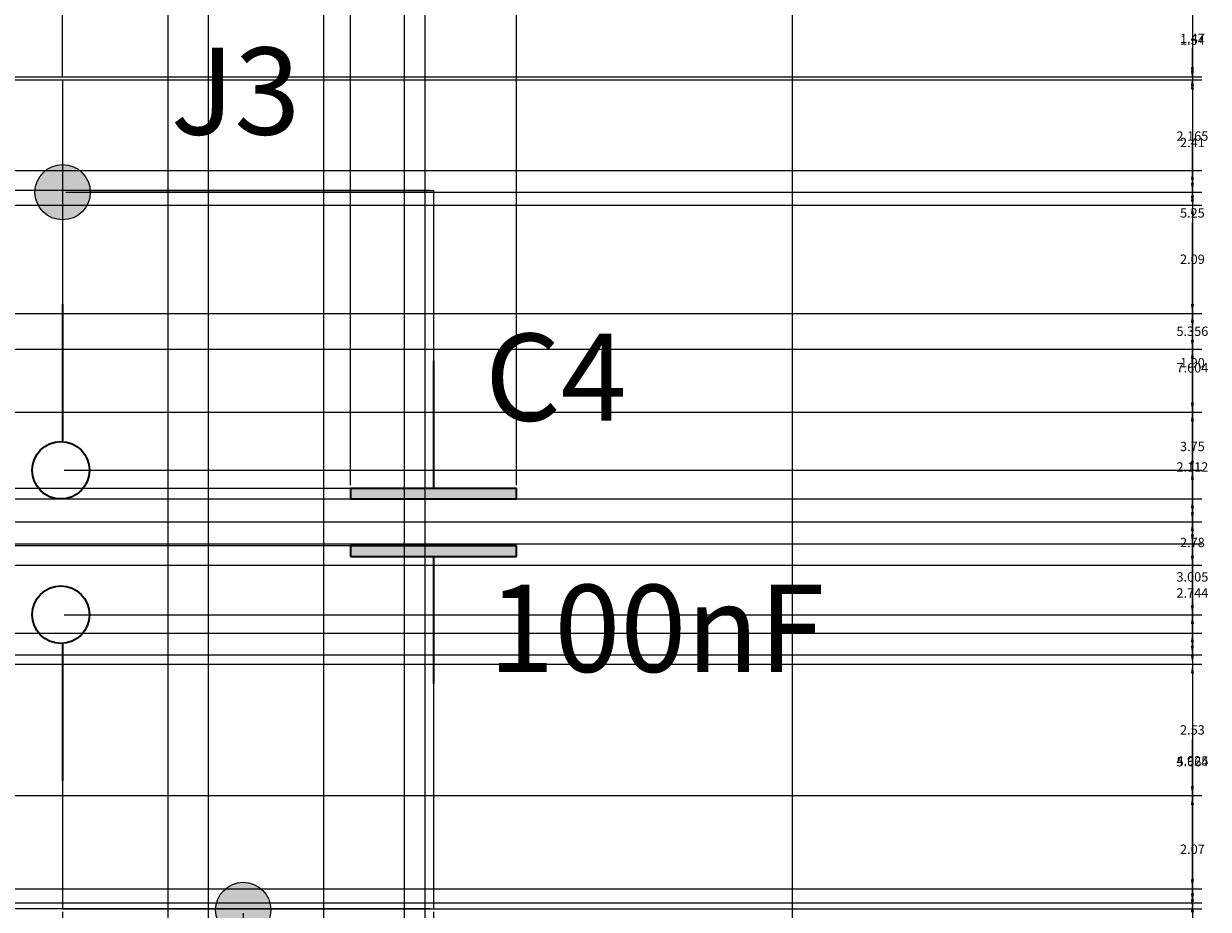
# Model space of a CAD drawing. Units: inches. Extents: x 23 to 132, y 5 to 105.
# Tile 12 of 14: x 106.54 to 129.37, y 59.58 to 76.64. Entities that reach past the tile are written whole.
import ezdxf

# ---------------------------------------------------------------- set-up
doc = ezdxf.new("R2010")
doc.units = ezdxf.units.IN
doc.header["$MEASUREMENT"] = 0
for name, color, linetype, lineweight in [('A-ANNO-DIMS', 2, 'Continuous', 18), ('E-ANNO-IDEN', 4, 'Continuous', 18), ('E-SYMB', 1, 'Continuous', 35), ('E-SYMB-PATT', 1, 'Continuous', 18), ('E-WIRE', 3, 'Continuous', 25), ('E-WIRE-PATT', 3, 'Continuous', 18)]:
    doc.layers.add(name, color=color, linetype=linetype, lineweight=lineweight)
doc.styles.get("Standard").update_dxf_attribs({"font": 'arial.ttf'})
doc.dimstyles.get("Standard").update_dxf_attribs({"dimtxt": 0.18, "dimasz": 0.18, "dimexe": 0.18, "dimexo": 0.0625, "dimgap": 0.09, "dimtad": 0, "dimtih": 1, "dimtoh": 1, "dimdec": 4, "dimzin": 0, "dimdsep": 46, "dimtxsty": 'Standard', "dimcen": 0.09, "dimadec": 0, "dimazin": 0, "dimtfac": 1, "dimtdec": 4, "dimtofl": 0, "dimtmove": 0, "dimatfit": 3, "dimfxl": 1, "dimtolj": 1, "dimtzin": 0, "dimarcsym": 0})

# ---------------------------------------------------------------- blocks, each defined once
blk = doc.blocks.new('*D2')
at = {"layer": 'A-ANNO-DIMS', "color": 0, "lineweight": -2, "transparency": 16777216}
for p, q in [((28.697, 66.272), (28.697, 105.232)), ((28.877, 105.052), (75.577, 105.052)), ((123.031, 105.052), (76.33, 105.052)), ((123.211, 99.539), (123.211, 105.232))]:
    blk.add_line(p, q, dxfattribs=at)
at = {"layer": 'A-ANNO-DIMS', "color": 0, "transparency": 16777216}
for points in [[(28.877, 105.082), (28.877, 105.022), (28.697, 105.052)], [(123.031, 105.082), (123.031, 105.022), (123.211, 105.052)]]:
    blk.add_solid(points, dxfattribs=at)
at = {"layer": 'Defpoints', "color": 0, "transparency": 16777216}
for p in [(123.211, 105.052), (123.211, 99.477), (28.697, 66.21)]:
    blk.add_point(p, dxfattribs=at)
at = {"layer": 'A-ANNO-DIMS', "color": 0, "transparency": 16777216, "insert": (75.954, 105.052), "char_height": 0.18, "attachment_point": 5}
blk.add_mtext('\\A1;94.51', dxfattribs=at)
blk = doc.blocks.new('*D3')
at = {"layer": 'A-ANNO-DIMS', "color": 0, "lineweight": -2, "transparency": 16777216}
for p, q in [((121.409, 99.285), (129.239, 99.285)), ((129.059, 99.105), (129.059, 55.423)), ((129.059, 11.378), (129.059, 55.06)), ((72.981, 11.198), (129.239, 11.198))]:
    blk.add_line(p, q, dxfattribs=at)
at = {"layer": 'A-ANNO-DIMS', "color": 0, "transparency": 16777216}
for points in [[(129.029, 99.105), (129.089, 99.105), (129.059, 99.285)], [(129.029, 11.378), (129.089, 11.378), (129.059, 11.198)]]:
    blk.add_solid(points, dxfattribs=at)
at = {"layer": 'Defpoints', "color": 0, "transparency": 16777216}
for p in [(121.346, 99.285), (129.059, 99.285), (72.919, 11.198)]:
    blk.add_point(p, dxfattribs=at)
at = {"layer": 'A-ANNO-DIMS', "color": 0, "transparency": 16777216, "insert": (129.059, 55.241), "char_height": 0.18, "attachment_point": 5}
blk.add_mtext('\\A1;88.09', dxfattribs=at)
blk = doc.blocks.new('*D15')
at = {"layer": 'A-ANNO-DIMS', "color": 0, "lineweight": -2, "transparency": 16777216}
for p, q in [((50.327, 77.095), (129.239, 77.095)), ((129.059, 76.915), (129.059, 76.538)), ((129.059, 75.801), (129.059, 76.177)), ((47.783, 75.621), (129.239, 75.621))]:
    blk.add_line(p, q, dxfattribs=at)
at = {"layer": 'A-ANNO-DIMS', "color": 0, "transparency": 16777216}
for points in [[(129.029, 76.915), (129.089, 76.915), (129.059, 77.095)], [(129.029, 75.801), (129.089, 75.801), (129.059, 75.621)]]:
    blk.add_solid(points, dxfattribs=at)
at = {"layer": 'Defpoints', "color": 0, "transparency": 16777216}
for p in [(50.265, 77.095), (47.72, 75.621), (129.059, 75.621)]:
    blk.add_point(p, dxfattribs=at)
at = {"layer": 'A-ANNO-DIMS', "color": 0, "transparency": 16777216, "insert": (129.059, 76.358), "char_height": 0.18, "attachment_point": 5}
blk.add_mtext('\\A1;1.47', dxfattribs=at)
blk = doc.blocks.new('*D16')
at = {"layer": 'A-ANNO-DIMS', "color": 0, "lineweight": -2, "transparency": 16777216}
for p, q in [((47.783, 75.621), (129.239, 75.621)), ((129.059, 75.441), (129.059, 73.177)), ((129.059, 70.55), (129.059, 72.814)), ((47.783, 70.37), (129.239, 70.37))]:
    blk.add_line(p, q, dxfattribs=at)
at = {"layer": 'A-ANNO-DIMS', "color": 0, "transparency": 16777216}
for points in [[(129.029, 75.441), (129.089, 75.441), (129.059, 75.621)], [(129.029, 70.55), (129.089, 70.55), (129.059, 70.37)]]:
    blk.add_solid(points, dxfattribs=at)
at = {"layer": 'Defpoints', "color": 0, "transparency": 16777216}
for p in [(47.72, 75.621), (47.72, 70.37), (129.059, 70.37)]:
    blk.add_point(p, dxfattribs=at)
at = {"layer": 'A-ANNO-DIMS', "color": 0, "transparency": 16777216, "insert": (129.059, 72.996), "char_height": 0.18, "attachment_point": 5}
blk.add_mtext('\\A1;5.25', dxfattribs=at)
blk = doc.blocks.new('*D17')
at = {"layer": 'A-ANNO-DIMS', "color": 0, "lineweight": -2, "transparency": 16777216}
for p, q in [((47.783, 70.37), (129.239, 70.37)), ((129.059, 70.19), (129.059, 68.678)), ((129.059, 66.801), (129.059, 68.314)), ((47.783, 66.621), (129.239, 66.621))]:
    blk.add_line(p, q, dxfattribs=at)
at = {"layer": 'A-ANNO-DIMS', "color": 0, "transparency": 16777216}
for points in [[(129.029, 70.19), (129.089, 70.19), (129.059, 70.37)], [(129.029, 66.801), (129.089, 66.801), (129.059, 66.621)]]:
    blk.add_solid(points, dxfattribs=at)
at = {"layer": 'Defpoints', "color": 0, "transparency": 16777216}
for p in [(47.72, 70.37), (47.72, 66.621), (129.059, 66.621)]:
    blk.add_point(p, dxfattribs=at)
at = {"layer": 'A-ANNO-DIMS', "color": 0, "transparency": 16777216, "insert": (129.059, 68.496), "char_height": 0.18, "attachment_point": 5}
blk.add_mtext('\\A1;3.75', dxfattribs=at)
blk = doc.blocks.new('*D24')
at = {"layer": 'A-ANNO-DIMS', "color": 0, "lineweight": -2, "transparency": 16777216}
for p, q in [((81.032, 77.095), (129.239, 77.095)), ((129.059, 76.915), (129.059, 76.509)), ((129.059, 75.739), (129.059, 76.145)), ((83.576, 75.559), (129.239, 75.559))]:
    blk.add_line(p, q, dxfattribs=at)
at = {"layer": 'A-ANNO-DIMS', "color": 0, "transparency": 16777216}
for points in [[(129.029, 76.915), (129.089, 76.915), (129.059, 77.095)], [(129.029, 75.739), (129.089, 75.739), (129.059, 75.559)]]:
    blk.add_solid(points, dxfattribs=at)
at = {"layer": 'Defpoints', "color": 0, "transparency": 16777216}
for p in [(80.969, 77.095), (83.514, 75.559), (129.059, 75.559)]:
    blk.add_point(p, dxfattribs=at)
at = {"layer": 'A-ANNO-DIMS', "color": 0, "transparency": 16777216, "insert": (129.059, 76.327), "char_height": 0.18, "attachment_point": 5}
blk.add_mtext('\\A1;1.54', dxfattribs=at)
blk = doc.blocks.new('*D25')
at = {"layer": 'A-ANNO-DIMS', "color": 0, "lineweight": -2, "transparency": 16777216}
for p, q in [((83.576, 75.559), (129.239, 75.559)), ((129.059, 75.379), (129.059, 74.534)), ((129.059, 73.327), (129.059, 74.173)), ((83.576, 73.147), (129.239, 73.147))]:
    blk.add_line(p, q, dxfattribs=at)
at = {"layer": 'A-ANNO-DIMS', "color": 0, "transparency": 16777216}
for points in [[(129.029, 75.379), (129.089, 75.379), (129.059, 75.559)], [(129.029, 73.327), (129.089, 73.327), (129.059, 73.147)]]:
    blk.add_solid(points, dxfattribs=at)
at = {"layer": 'Defpoints', "color": 0, "transparency": 16777216}
for p in [(83.514, 75.559), (83.514, 73.147), (129.059, 73.147)]:
    blk.add_point(p, dxfattribs=at)
at = {"layer": 'A-ANNO-DIMS', "color": 0, "transparency": 16777216, "insert": (129.059, 74.353), "char_height": 0.18, "attachment_point": 5}
blk.add_mtext('\\A1;2.41', dxfattribs=at)
blk = doc.blocks.new('*D26')
at = {"layer": 'A-ANNO-DIMS', "color": 0, "lineweight": -2, "transparency": 16777216}
for p, q in [((83.576, 73.147), (129.239, 73.147)), ((129.059, 72.967), (129.059, 72.286)), ((129.059, 71.241), (129.059, 71.922)), ((83.576, 71.061), (129.239, 71.061))]:
    blk.add_line(p, q, dxfattribs=at)
at = {"layer": 'A-ANNO-DIMS', "color": 0, "transparency": 16777216}
for points in [[(129.029, 72.967), (129.089, 72.967), (129.059, 73.147)], [(129.029, 71.241), (129.089, 71.241), (129.059, 71.061)]]:
    blk.add_solid(points, dxfattribs=at)
at = {"layer": 'Defpoints', "color": 0, "transparency": 16777216}
for p in [(83.514, 73.147), (83.514, 71.061), (129.059, 71.061)]:
    blk.add_point(p, dxfattribs=at)
at = {"layer": 'A-ANNO-DIMS', "color": 0, "transparency": 16777216, "insert": (129.059, 72.104), "char_height": 0.18, "attachment_point": 5}
blk.add_mtext('\\A1;2.09', dxfattribs=at)
blk = doc.blocks.new('*D27')
at = {"layer": 'A-ANNO-DIMS', "color": 0, "lineweight": -2, "transparency": 16777216}
for p, q in [((83.576, 71.061), (129.239, 71.061)), ((129.059, 70.881), (129.059, 70.292)), ((129.059, 69.338), (129.059, 69.928)), ((83.576, 69.158), (129.239, 69.158))]:
    blk.add_line(p, q, dxfattribs=at)
at = {"layer": 'A-ANNO-DIMS', "color": 0, "transparency": 16777216}
for points in [[(129.029, 70.881), (129.089, 70.881), (129.059, 71.061)], [(129.029, 69.338), (129.089, 69.338), (129.059, 69.158)]]:
    blk.add_solid(points, dxfattribs=at)
at = {"layer": 'Defpoints', "color": 0, "transparency": 16777216}
for p in [(83.514, 71.061), (83.514, 69.158), (129.059, 69.158)]:
    blk.add_point(p, dxfattribs=at)
at = {"layer": 'A-ANNO-DIMS', "color": 0, "transparency": 16777216, "insert": (129.059, 70.11), "char_height": 0.18, "attachment_point": 5}
blk.add_mtext('\\A1;1.90', dxfattribs=at)
blk = doc.blocks.new('*D28')
at = {"layer": 'A-ANNO-DIMS', "color": 0, "lineweight": -2, "transparency": 16777216}
for p, q in [((83.576, 69.158), (129.239, 69.158)), ((129.059, 68.978), (129.059, 68.282)), ((129.059, 67.226), (129.059, 67.922)), ((83.576, 67.046), (129.239, 67.046))]:
    blk.add_line(p, q, dxfattribs=at)
at = {"layer": 'A-ANNO-DIMS', "color": 0, "transparency": 16777216}
for points in [[(129.029, 68.978), (129.089, 68.978), (129.059, 69.158)], [(129.029, 67.226), (129.089, 67.226), (129.059, 67.046)]]:
    blk.add_solid(points, dxfattribs=at)
at = {"layer": 'Defpoints', "color": 0, "transparency": 16777216}
for p in [(83.514, 69.158), (83.514, 67.046), (129.059, 67.046)]:
    blk.add_point(p, dxfattribs=at)
at = {"layer": 'A-ANNO-DIMS', "color": 0, "transparency": 16777216, "insert": (129.059, 68.102), "char_height": 0.18, "attachment_point": 5}
blk.add_mtext('\\A1;2.112', dxfattribs=at)
blk = doc.blocks.new('*D29')
at = {"layer": 'A-ANNO-DIMS', "color": 0, "lineweight": -2, "transparency": 16777216}
for p, q in [((83.576, 67.046), (129.239, 67.046)), ((129.059, 66.866), (129.059, 65.855)), ((129.059, 64.482), (129.059, 65.494)), ((83.576, 64.302), (129.239, 64.302))]:
    blk.add_line(p, q, dxfattribs=at)
at = {"layer": 'A-ANNO-DIMS', "color": 0, "transparency": 16777216}
for points in [[(129.029, 66.866), (129.089, 66.866), (129.059, 67.046)], [(129.029, 64.482), (129.089, 64.482), (129.059, 64.302)]]:
    blk.add_solid(points, dxfattribs=at)
at = {"layer": 'Defpoints', "color": 0, "transparency": 16777216}
for p in [(83.514, 67.046), (83.514, 64.302), (129.059, 64.302)]:
    blk.add_point(p, dxfattribs=at)
at = {"layer": 'A-ANNO-DIMS', "color": 0, "transparency": 16777216, "insert": (129.059, 65.674), "char_height": 0.18, "attachment_point": 5}
blk.add_mtext('\\A1;2.744', dxfattribs=at)
blk = doc.blocks.new('*D30')
at = {"layer": 'A-ANNO-DIMS', "color": 0, "lineweight": -2, "transparency": 16777216}
for p, q in [((83.576, 64.302), (129.239, 64.302)), ((129.059, 64.122), (129.059, 63.217)), ((129.059, 61.949), (129.059, 62.853)), ((83.576, 61.769), (129.239, 61.769))]:
    blk.add_line(p, q, dxfattribs=at)
at = {"layer": 'A-ANNO-DIMS', "color": 0, "transparency": 16777216}
for points in [[(129.029, 64.122), (129.089, 64.122), (129.059, 64.302)], [(129.029, 61.949), (129.089, 61.949), (129.059, 61.769)]]:
    blk.add_solid(points, dxfattribs=at)
at = {"layer": 'Defpoints', "color": 0, "transparency": 16777216}
for p in [(83.514, 64.302), (83.514, 61.769), (129.059, 61.769)]:
    blk.add_point(p, dxfattribs=at)
at = {"layer": 'A-ANNO-DIMS', "color": 0, "transparency": 16777216, "insert": (129.059, 63.035), "char_height": 0.18, "attachment_point": 5}
blk.add_mtext('\\A1;2.53', dxfattribs=at)
blk = doc.blocks.new('*D31')
at = {"layer": 'A-ANNO-DIMS', "color": 0, "lineweight": -2, "transparency": 16777216}
for p, q in [((83.576, 61.769), (129.239, 61.769)), ((129.059, 61.589), (129.059, 60.918)), ((129.059, 59.883), (129.059, 60.554)), ((83.576, 59.703), (129.239, 59.703))]:
    blk.add_line(p, q, dxfattribs=at)
at = {"layer": 'A-ANNO-DIMS', "color": 0, "transparency": 16777216}
for points in [[(129.029, 61.589), (129.089, 61.589), (129.059, 61.769)], [(129.029, 59.883), (129.089, 59.883), (129.059, 59.703)]]:
    blk.add_solid(points, dxfattribs=at)
at = {"layer": 'Defpoints', "color": 0, "transparency": 16777216}
for p in [(83.514, 61.769), (83.514, 59.703), (129.059, 59.703)]:
    blk.add_point(p, dxfattribs=at)
at = {"layer": 'A-ANNO-DIMS', "color": 0, "transparency": 16777216, "insert": (129.059, 60.736), "char_height": 0.18, "attachment_point": 5}
blk.add_mtext('\\A1;2.07', dxfattribs=at)
blk = doc.blocks.new('*D32')
at = {"layer": 'A-ANNO-DIMS', "color": 0, "lineweight": -2, "transparency": 16777216}
for p, q in [((83.576, 59.703), (129.239, 59.703)), ((129.059, 59.523), (129.059, 58.629)), ((129.059, 57.372), (129.059, 58.266)), ((83.576, 57.192), (129.239, 57.192))]:
    blk.add_line(p, q, dxfattribs=at)
at = {"layer": 'A-ANNO-DIMS', "color": 0, "transparency": 16777216}
for points in [[(129.029, 59.523), (129.089, 59.523), (129.059, 59.703)], [(129.029, 57.372), (129.089, 57.372), (129.059, 57.192)]]:
    blk.add_solid(points, dxfattribs=at)
at = {"layer": 'Defpoints', "color": 0, "transparency": 16777216}
for p in [(83.514, 59.703), (83.514, 57.192), (129.059, 57.192)]:
    blk.add_point(p, dxfattribs=at)
at = {"layer": 'A-ANNO-DIMS', "color": 0, "transparency": 16777216, "insert": (129.059, 58.447), "char_height": 0.18, "attachment_point": 5}
blk.add_mtext('\\A1;2.51', dxfattribs=at)
blk = doc.blocks.new('*D49')
at = {"layer": 'A-ANNO-DIMS', "color": 0, "lineweight": -2, "transparency": 16777216}
for p, q in [((83.514, 75.622), (83.514, 105.232)), ((83.694, 105.052), (94.936, 105.052)), ((107.107, 105.052), (95.865, 105.052)), ((107.287, 75.622), (107.287, 105.232))]:
    blk.add_line(p, q, dxfattribs=at)
at = {"layer": 'A-ANNO-DIMS', "color": 0, "transparency": 16777216}
for points in [[(83.694, 105.082), (83.694, 105.022), (83.514, 105.052)], [(107.107, 105.082), (107.107, 105.022), (107.287, 105.052)]]:
    blk.add_solid(points, dxfattribs=at)
at = {"layer": 'Defpoints', "color": 0, "transparency": 16777216}
for p in [(107.287, 105.052), (83.514, 75.559), (107.287, 75.559)]:
    blk.add_point(p, dxfattribs=at)
at = {"layer": 'A-ANNO-DIMS', "color": 0, "transparency": 16777216, "insert": (95.4, 105.052), "char_height": 0.18, "attachment_point": 5}
blk.add_mtext('\\A1;23.774', dxfattribs=at)
blk = doc.blocks.new('*D57')
at = {"layer": 'A-ANNO-DIMS', "color": 0, "lineweight": -2, "transparency": 16777216}
for p, q in [((30.358, 64.901), (129.239, 64.901)), ((129.059, 64.721), (129.059, 62.62)), ((129.059, 60.155), (129.059, 62.256)), ((30.358, 59.975), (129.239, 59.975))]:
    blk.add_line(p, q, dxfattribs=at)
at = {"layer": 'A-ANNO-DIMS', "color": 0, "transparency": 16777216}
for points in [[(129.029, 64.721), (129.089, 64.721), (129.059, 64.901)], [(129.029, 60.155), (129.089, 60.155), (129.059, 59.975)]]:
    blk.add_solid(points, dxfattribs=at)
at = {"layer": 'Defpoints', "color": 0, "transparency": 16777216}
for p in [(30.295, 64.901), (129.059, 64.901), (30.295, 59.975)]:
    blk.add_point(p, dxfattribs=at)
at = {"layer": 'A-ANNO-DIMS', "color": 0, "transparency": 16777216, "insert": (129.059, 62.438), "char_height": 0.18, "attachment_point": 5}
blk.add_mtext('\\A1;4.925', dxfattribs=at)
blk = doc.blocks.new('*D58')
at = {"layer": 'A-ANNO-DIMS', "color": 0, "lineweight": -2, "transparency": 16777216}
for p, q in [((30.358, 73.814), (129.239, 73.814)), ((129.059, 73.634), (129.059, 70.194)), ((129.059, 66.39), (129.059, 69.83)), ((30.359, 66.21), (129.239, 66.21))]:
    blk.add_line(p, q, dxfattribs=at)
at = {"layer": 'A-ANNO-DIMS', "color": 0, "transparency": 16777216}
for points in [[(129.029, 73.634), (129.089, 73.634), (129.059, 73.814)], [(129.029, 66.39), (129.089, 66.39), (129.059, 66.21)]]:
    blk.add_solid(points, dxfattribs=at)
at = {"layer": 'Defpoints', "color": 0, "transparency": 16777216}
for p in [(30.295, 73.814), (129.059, 73.814), (30.297, 66.21)]:
    blk.add_point(p, dxfattribs=at)
at = {"layer": 'A-ANNO-DIMS', "color": 0, "transparency": 16777216, "insert": (129.059, 70.012), "char_height": 0.18, "attachment_point": 5}
blk.add_mtext('\\A1;7.604', dxfattribs=at)
blk = doc.blocks.new('*D65')
at = {"layer": 'A-ANNO-DIMS', "color": 0, "lineweight": -2, "transparency": 16777216}
for p, q in [((38.414, 67.485), (129.239, 67.485)), ((129.059, 67.305), (129.059, 66.165)), ((129.059, 64.66), (129.059, 65.801)), ((38.414, 64.48), (129.239, 64.48))]:
    blk.add_line(p, q, dxfattribs=at)
at = {"layer": 'A-ANNO-DIMS', "color": 0, "transparency": 16777216}
for points in [[(129.029, 67.305), (129.089, 67.305), (129.059, 67.485)], [(129.029, 64.66), (129.089, 64.66), (129.059, 64.48)]]:
    blk.add_solid(points, dxfattribs=at)
at = {"layer": 'Defpoints', "color": 0, "transparency": 16777216}
for p in [(38.351, 67.485), (129.059, 67.485), (38.351, 64.48)]:
    blk.add_point(p, dxfattribs=at)
at = {"layer": 'A-ANNO-DIMS', "color": 0, "transparency": 16777216, "insert": (129.059, 65.983), "char_height": 0.18, "attachment_point": 5}
blk.add_mtext('\\A1;3.005', dxfattribs=at)
blk = doc.blocks.new('*D71')
at = {"layer": 'A-ANNO-DIMS', "color": 0, "lineweight": -2, "transparency": 16777216}
for p, q in [((107.316, 65.255), (129.239, 65.255)), ((129.059, 65.075), (129.059, 62.604)), ((129.059, 59.77), (129.059, 62.241)), ((107.35, 59.59), (129.239, 59.59))]:
    blk.add_line(p, q, dxfattribs=at)
at = {"layer": 'A-ANNO-DIMS', "color": 0, "transparency": 16777216}
for points in [[(129.029, 65.075), (129.089, 65.075), (129.059, 65.255)], [(129.029, 59.77), (129.089, 59.77), (129.059, 59.59)]]:
    blk.add_solid(points, dxfattribs=at)
at = {"layer": 'Defpoints', "color": 0, "transparency": 16777216}
for p in [(107.253, 65.255), (129.059, 65.255), (107.287, 59.59)]:
    blk.add_point(p, dxfattribs=at)
at = {"layer": 'A-ANNO-DIMS', "color": 0, "transparency": 16777216, "insert": (129.059, 62.422), "char_height": 0.18, "attachment_point": 5}
blk.add_mtext('\\A1;5.664', dxfattribs=at)
blk = doc.blocks.new('*D72')
at = {"layer": 'A-ANNO-DIMS', "color": 0, "lineweight": -2, "transparency": 16777216}
for p, q in [((107.316, 68.038), (129.239, 68.038)), ((129.059, 67.858), (129.059, 66.828)), ((129.059, 65.435), (129.059, 66.464)), ((107.316, 65.255), (129.239, 65.255))]:
    blk.add_line(p, q, dxfattribs=at)
at = {"layer": 'A-ANNO-DIMS', "color": 0, "transparency": 16777216}
for points in [[(129.029, 67.858), (129.089, 67.858), (129.059, 68.038)], [(129.029, 65.435), (129.089, 65.435), (129.059, 65.255)]]:
    blk.add_solid(points, dxfattribs=at)
at = {"layer": 'Defpoints', "color": 0, "transparency": 16777216}
for p in [(107.253, 68.038), (129.059, 68.038), (107.253, 65.255)]:
    blk.add_point(p, dxfattribs=at)
at = {"layer": 'A-ANNO-DIMS', "color": 0, "transparency": 16777216, "insert": (129.059, 66.646), "char_height": 0.18, "attachment_point": 5}
blk.add_mtext('\\A1;2.78', dxfattribs=at)
blk = doc.blocks.new('*D73')
at = {"layer": 'A-ANNO-DIMS', "color": 0, "lineweight": -2, "transparency": 16777216}
for p, q in [((107.35, 73.395), (129.239, 73.395)), ((129.059, 73.215), (129.059, 70.898)), ((129.059, 68.218), (129.059, 70.534)), ((107.316, 68.038), (129.239, 68.038))]:
    blk.add_line(p, q, dxfattribs=at)
at = {"layer": 'A-ANNO-DIMS', "color": 0, "transparency": 16777216}
for points in [[(129.029, 73.215), (129.089, 73.215), (129.059, 73.395)], [(129.029, 68.218), (129.089, 68.218), (129.059, 68.038)]]:
    blk.add_solid(points, dxfattribs=at)
at = {"layer": 'Defpoints', "color": 0, "transparency": 16777216}
for p in [(107.287, 73.395), (129.059, 73.395), (107.253, 68.038)]:
    blk.add_point(p, dxfattribs=at)
at = {"layer": 'A-ANNO-DIMS', "color": 0, "transparency": 16777216, "insert": (129.059, 70.716), "char_height": 0.18, "attachment_point": 5}
blk.add_mtext('\\A1;5.356', dxfattribs=at)
blk = doc.blocks.new('*D74')
at = {"layer": 'A-ANNO-DIMS', "color": 0, "lineweight": -2, "transparency": 16777216}
for p, q in [((107.35, 75.559), (129.239, 75.559)), ((129.059, 75.379), (129.059, 74.659)), ((129.059, 73.575), (129.059, 74.295)), ((107.35, 73.395), (129.239, 73.395))]:
    blk.add_line(p, q, dxfattribs=at)
at = {"layer": 'A-ANNO-DIMS', "color": 0, "transparency": 16777216}
for points in [[(129.029, 75.379), (129.089, 75.379), (129.059, 75.559)], [(129.029, 73.575), (129.089, 73.575), (129.059, 73.395)]]:
    blk.add_solid(points, dxfattribs=at)
at = {"layer": 'Defpoints', "color": 0, "transparency": 16777216}
for p in [(107.287, 75.559), (129.059, 75.559), (107.287, 73.395)]:
    blk.add_point(p, dxfattribs=at)
at = {"layer": 'A-ANNO-DIMS', "color": 0, "transparency": 16777216, "insert": (129.059, 74.477), "char_height": 0.18, "attachment_point": 5}
blk.add_mtext('\\A1;2.165', dxfattribs=at)
blk = doc.blocks.new('*D75')
at = {"layer": 'A-ANNO-DIMS', "color": 0, "lineweight": -2, "transparency": 16777216}
for p, q in [((107.287, 59.528), (107.287, 5.443)), ((110.768, 59.503), (110.768, 5.443)), ((107.467, 5.623), (108.704, 5.623)), ((110.588, 5.623), (109.351, 5.623))]:
    blk.add_line(p, q, dxfattribs=at)
at = {"layer": 'A-ANNO-DIMS', "color": 0, "transparency": 16777216}
for points in [[(107.467, 5.653), (107.467, 5.593), (107.287, 5.623)], [(110.588, 5.653), (110.588, 5.593), (110.768, 5.623)]]:
    blk.add_solid(points, dxfattribs=at)
at = {"layer": 'Defpoints', "color": 0, "transparency": 16777216}
for p in [(107.287, 59.59), (110.768, 59.566), (110.768, 5.623)]:
    blk.add_point(p, dxfattribs=at)
at = {"layer": 'A-ANNO-DIMS', "color": 0, "transparency": 16777216, "insert": (109.028, 5.623), "char_height": 0.18, "attachment_point": 5}
blk.add_mtext('\\A1;3.48', dxfattribs=at)
blk = doc.blocks.new('*D76')
at = {"layer": 'A-ANNO-DIMS', "color": 0, "lineweight": -2, "transparency": 16777216}
for p, q in [((110.768, 59.503), (110.768, 5.443)), ((114.434, 59.528), (114.434, 5.443)), ((110.948, 5.623), (112.207, 5.623)), ((114.254, 5.623), (112.994, 5.623))]:
    blk.add_line(p, q, dxfattribs=at)
at = {"layer": 'A-ANNO-DIMS', "color": 0, "transparency": 16777216}
for points in [[(110.948, 5.653), (110.948, 5.593), (110.768, 5.623)], [(114.254, 5.653), (114.254, 5.593), (114.434, 5.623)]]:
    blk.add_solid(points, dxfattribs=at)
at = {"layer": 'Defpoints', "color": 0, "transparency": 16777216}
for p in [(114.434, 59.59), (110.768, 59.566), (114.434, 5.623)]:
    blk.add_point(p, dxfattribs=at)
at = {"layer": 'A-ANNO-DIMS', "color": 0, "transparency": 16777216, "insert": (112.601, 5.623), "char_height": 0.18, "attachment_point": 5}
blk.add_mtext('\\A1;3.666', dxfattribs=at)
blk = doc.blocks.new('*D77')
at = {"layer": 'A-ANNO-DIMS', "color": 0, "lineweight": -2, "transparency": 16777216}
for p, q in [((112.835, 67.751), (112.835, 105.232)), ((113.015, 105.052), (114.182, 105.052)), ((115.855, 105.052), (114.688, 105.052)), ((116.035, 67.751), (116.035, 105.232))]:
    blk.add_line(p, q, dxfattribs=at)
at = {"layer": 'A-ANNO-DIMS', "color": 0, "transparency": 16777216}
for points in [[(113.015, 105.082), (113.015, 105.022), (112.835, 105.052)], [(115.855, 105.082), (115.855, 105.022), (116.035, 105.052)]]:
    blk.add_solid(points, dxfattribs=at)
at = {"layer": 'Defpoints', "color": 0, "transparency": 16777216}
for p in [(116.035, 105.052), (112.835, 67.688), (116.035, 67.688)]:
    blk.add_point(p, dxfattribs=at)
at = {"layer": 'A-ANNO-DIMS', "color": 0, "transparency": 16777216, "insert": (114.435, 105.052), "char_height": 0.18, "attachment_point": 5}
blk.add_mtext('\\A1;3.2', dxfattribs=at)
blk = doc.blocks.new('*D78')
at = {"layer": 'A-ANNO-DIMS', "color": 0, "lineweight": -2, "transparency": 16777216}
for p, q in [((112.773, 67.688), (22.942, 67.688)), ((23.122, 67.508), (23.122, 67.314)), ((23.122, 66.759), (23.122, 66.953)), ((112.773, 66.579), (22.942, 66.579))]:
    blk.add_line(p, q, dxfattribs=at)
at = {"layer": 'A-ANNO-DIMS', "color": 0, "transparency": 16777216}
for points in [[(23.092, 67.508), (23.152, 67.508), (23.122, 67.688)], [(23.092, 66.759), (23.152, 66.759), (23.122, 66.579)]]:
    blk.add_solid(points, dxfattribs=at)
at = {"layer": 'Defpoints', "color": 0, "transparency": 16777216}
for p in [(23.122, 67.688), (112.835, 67.688), (112.835, 66.579)]:
    blk.add_point(p, dxfattribs=at)
at = {"layer": 'A-ANNO-DIMS', "color": 0, "transparency": 16777216, "insert": (23.122, 67.133), "char_height": 0.18, "attachment_point": 5}
blk.add_mtext('\\A1;1.11', dxfattribs=at)
blk = doc.blocks.new('*D79')
at = {"layer": 'A-ANNO-DIMS', "color": 0, "lineweight": -2, "transparency": 16777216}
for p, q in [((114.373, 66.579), (22.942, 66.579)), ((23.122, 66.399), (23.122, 63.267)), ((23.122, 59.77), (23.122, 62.903)), ((114.371, 59.59), (22.942, 59.59))]:
    blk.add_line(p, q, dxfattribs=at)
at = {"layer": 'A-ANNO-DIMS', "color": 0, "transparency": 16777216}
for points in [[(23.092, 66.399), (23.152, 66.399), (23.122, 66.579)], [(23.092, 59.77), (23.152, 59.77), (23.122, 59.59)]]:
    blk.add_solid(points, dxfattribs=at)
at = {"layer": 'Defpoints', "color": 0, "transparency": 16777216}
for p in [(23.122, 66.579), (114.435, 66.579), (114.434, 59.59)]:
    blk.add_point(p, dxfattribs=at)
at = {"layer": 'A-ANNO-DIMS', "color": 0, "transparency": 16777216, "insert": (23.122, 63.085), "char_height": 0.18, "attachment_point": 5}
blk.add_mtext('\\A1;6.988', dxfattribs=at)
blk = doc.blocks.new('*D80')
at = {"layer": 'A-ANNO-DIMS', "color": 0, "lineweight": -2, "transparency": 16777216}
for p, q in [((114.373, 73.429), (22.942, 73.429)), ((23.122, 73.249), (23.122, 70.741)), ((23.122, 67.868), (23.122, 70.377)), ((114.373, 67.688), (22.942, 67.688))]:
    blk.add_line(p, q, dxfattribs=at)
at = {"layer": 'A-ANNO-DIMS', "color": 0, "transparency": 16777216}
for points in [[(23.092, 73.249), (23.152, 73.249), (23.122, 73.429)], [(23.092, 67.868), (23.152, 67.868), (23.122, 67.688)]]:
    blk.add_solid(points, dxfattribs=at)
at = {"layer": 'Defpoints', "color": 0, "transparency": 16777216}
for p in [(23.122, 73.429), (114.435, 73.429), (114.435, 67.688)]:
    blk.add_point(p, dxfattribs=at)
at = {"layer": 'A-ANNO-DIMS', "color": 0, "transparency": 16777216, "insert": (23.122, 70.559), "char_height": 0.18, "attachment_point": 5}
blk.add_mtext('\\A1;5.741', dxfattribs=at)
blk = doc.blocks.new('*D82')
at = {"layer": 'A-ANNO-DIMS', "color": 0, "lineweight": -2, "transparency": 16777216}
for p, q in [((109.322, 56.302), (109.322, 105.232)), ((109.502, 105.052), (110.673, 105.052)), ((112.142, 105.052), (110.971, 105.052)), ((112.322, 56.302), (112.322, 105.232))]:
    blk.add_line(p, q, dxfattribs=at)
at = {"layer": 'A-ANNO-DIMS', "color": 0, "transparency": 16777216}
for points in [[(109.502, 105.082), (109.502, 105.022), (109.322, 105.052)], [(112.142, 105.082), (112.142, 105.022), (112.322, 105.052)]]:
    blk.add_solid(points, dxfattribs=at)
at = {"layer": 'Defpoints', "color": 0, "transparency": 16777216}
for p in [(112.322, 105.052), (109.322, 56.24), (112.322, 56.24)]:
    blk.add_point(p, dxfattribs=at)
at = {"layer": 'A-ANNO-DIMS', "color": 0, "transparency": 16777216, "insert": (110.822, 105.052), "char_height": 0.18, "attachment_point": 5}
blk.add_mtext('\\A1;3', dxfattribs=at)
blk = doc.blocks.new('*D91')
at = {"layer": 'A-ANNO-DIMS', "color": 0, "lineweight": -2, "transparency": 16777216}
for p, q in [((110.089, 79.853), (110.089, 5.443)), ((113.872, 79.853), (113.872, 5.443)), ((110.269, 5.623), (111.587, 5.623)), ((113.692, 5.623), (112.374, 5.623))]:
    blk.add_line(p, q, dxfattribs=at)
at = {"layer": 'A-ANNO-DIMS', "color": 0, "transparency": 16777216}
for points in [[(110.269, 5.653), (110.269, 5.593), (110.089, 5.623)], [(113.692, 5.653), (113.692, 5.593), (113.872, 5.623)]]:
    blk.add_solid(points, dxfattribs=at)
at = {"layer": 'Defpoints', "color": 0, "transparency": 16777216}
for p in [(110.089, 79.916), (113.872, 79.916), (113.872, 5.623)]:
    blk.add_point(p, dxfattribs=at)
at = {"layer": 'A-ANNO-DIMS', "color": 0, "transparency": 16777216, "insert": (111.981, 5.623), "char_height": 0.18, "attachment_point": 5}
blk.add_mtext('\\A1;3.783', dxfattribs=at)
blk = doc.blocks.new('*D93')
at = {"layer": 'A-ANNO-DIMS', "color": 0, "lineweight": -2, "transparency": 16777216}
for p, q in [((114.269, 94.721), (114.269, 5.443)), ((121.346, 94.721), (121.346, 5.443)), ((114.449, 5.623), (117.415, 5.623)), ((121.166, 5.623), (118.201, 5.623))]:
    blk.add_line(p, q, dxfattribs=at)
at = {"layer": 'A-ANNO-DIMS', "color": 0, "transparency": 16777216}
for points in [[(114.449, 5.653), (114.449, 5.593), (114.269, 5.623)], [(121.166, 5.653), (121.166, 5.593), (121.346, 5.623)]]:
    blk.add_solid(points, dxfattribs=at)
at = {"layer": 'Defpoints', "color": 0, "transparency": 16777216}
for p in [(114.269, 94.783), (121.346, 94.783), (121.346, 5.623)]:
    blk.add_point(p, dxfattribs=at)
at = {"layer": 'A-ANNO-DIMS', "color": 0, "transparency": 16777216, "insert": (117.808, 5.623), "char_height": 0.18, "attachment_point": 5}
blk.add_mtext('\\A1;7.077', dxfattribs=at)

msp = doc.modelspace()

# ---------------------------------------------------------------- hatches: boundary and pattern name
at = {"layer": 'E-SYMB-PATT'}
h = msp.add_hatch(color=256, dxfattribs=at)
h.dxf.hatch_style = 1
h.paths.add_polyline_path([(112.8351, 67.6881), (112.8351, 67.4881), (116.0351, 67.4881), (116.0351, 67.6881), (114.4351, 67.6881)])
h.paths.add_polyline_path([(116.0351, 66.3788), (116.0351, 66.5788), (114.4351, 66.5788), (112.8351, 66.5788), (112.8351, 66.3788)])
at = {"layer": 'E-WIRE-PATT'}
h = msp.add_hatch(color=256, dxfattribs=at)
h.dxf.hatch_style = 1
h.paths.add_polyline_path([(107.8201, 73.3945, 0.4142136), (107.2874, 73.9273), (107.2874, 72.8618, 0.4142136)])
h.paths.add_polyline_path([(107.2874, 73.9273, 0.4142136), (106.7546, 73.3945, 0.4142136), (107.2874, 72.8618)])
h.paths.add_polyline_path([(110.2355, 59.5904), (111.2999, 59.5904, 0.9551697)])
h.paths.add_polyline_path([(111.3005, 59.566, 0.011463), (111.2999, 59.5904), (110.2355, 59.5904, 0.011463), (110.235, 59.566, 1)])

# ---------------------------------------------------------------- linework, layer by layer
at = {"layer": 'E-SYMB'}
for p, q in [((107.2874, 71.2363), (107.2874, 68.5907)), ((114.4351, 70.1475), (114.4351, 67.6881)), ((114.4351, 67.6881), (112.8351, 67.6881)), ((112.8351, 67.6881), (112.8351, 67.4881)), ((116.0351, 67.6881), (114.4351, 67.6881)), ((116.0351, 67.4881), (116.0351, 67.6881)), ((112.8351, 67.4881), (116.0351, 67.4881)), ((114.4351, 66.5788), (112.8351, 66.5788)), ((112.8351, 66.5788), (112.8351, 66.3788)), ((116.0351, 66.5788), (114.4351, 66.5788)), ((116.0351, 66.3788), (116.0351, 66.5788)), ((112.8351, 66.3788), (116.0351, 66.3788)), ((114.434, 66.3788), (114.434, 63.9194)), ((107.2829, 64.7018), (107.2829, 62.0562))]:
    msp.add_line(p, q, dxfattribs=at)
for centre in [(107.253, 68.0382), (107.253, 65.2546)]:
    msp.add_circle(centre, 0.5536, dxfattribs=at)
at = {"layer": 'E-WIRE'}
for p, q in [((94.2651, 75.5594), (107.2874, 75.5594)), ((107.2874, 75.5594), (107.2874, 71.2363)), ((107.819, 73.4293), (114.4351, 73.4293)), ((114.4351, 73.4293), (114.4351, 70.1475)), ((114.434, 63.9194), (114.434, 59.5904)), ((107.2874, 62.0562), (107.2874, 59.5904)), ((107.2874, 59.5904), (114.434, 59.5904))]:
    msp.add_line(p, q, dxfattribs=at)
for centre in [(107.2874, 73.3945), (110.7677, 59.566)]:
    msp.add_circle(centre, 0.5327, dxfattribs=at)

# ---------------------------------------------------------------- texts
at = {"layer": 'E-ANNO-IDEN'}
for s, p in [('J3', (109.3704, 74.5035)), ('C4', (115.4254, 68.9912)), ('100nF', (115.4926, 64.1512))]:
    msp.add_text(s, height=1.67943, dxfattribs=at).set_placement(p)

# ---------------------------------------------------------------- dimensions: what is measured, and where the dimension line sits
at = {"layer": 'A-ANNO-DIMS'}
for base, p1, p2, override, picture, middle in [((123.2107, 105.052), (28.6965, 66.2099), (123.2107, 99.477), {"dimdec": 2, "dimlfac": 1, "dimrnd": 0, "dimzin": 0, "dimdsep": 46, "dimlunit": 2}, '*D2', (75.9536, 105.052)), ((107.2874, 105.052), (83.5136, 75.5594), (107.2874, 75.5594), {"dimdec": 3, "dimlfac": 1, "dimrnd": 0, "dimzin": 0, "dimdsep": 46, "dimlunit": 2}, '*D49', (95.4005, 105.052)), ((112.3219, 105.052), (109.3219, 56.2399), (112.3219, 56.2399), {"dimdec": 0, "dimlfac": 1, "dimrnd": 0, "dimzin": 0, "dimdsep": 46, "dimlunit": 2}, '*D82', (110.8219, 105.052)), ((116.0351, 105.052), (112.8351, 67.6881), (116.0351, 67.6881), {"dimdec": 1, "dimlfac": 1, "dimrnd": 0, "dimzin": 0, "dimdsep": 46, "dimlunit": 2}, '*D77', (114.4351, 105.052)), ((121.3461, 5.6233), (114.2693, 94.7833), (121.3461, 94.7833), {"dimdec": 3, "dimlfac": 1, "dimrnd": 0, "dimzin": 0, "dimdsep": 46, "dimlunit": 2}, '*D93', (117.8077, 5.6233)), ((113.8719, 5.6233), (110.0892, 79.9158), (113.8719, 79.9158), {"dimdec": 3, "dimlfac": 1, "dimrnd": 0, "dimzin": 0, "dimdsep": 46, "dimlunit": 2}, '*D91', (111.9805, 5.6233)), ((110.7677, 5.6233), (107.2874, 59.5904), (110.7677, 59.566), {"dimdec": 2, "dimlfac": 1, "dimrnd": 0, "dimzin": 0, "dimdsep": 46, "dimlunit": 2}, '*D75', (109.0275, 5.6233)), ((114.434, 5.6233), (110.7677, 59.566), (114.434, 59.5904), {"dimdec": 3, "dimlfac": 1, "dimrnd": 0, "dimzin": 0, "dimdsep": 46, "dimlunit": 2}, '*D76', (112.6009, 5.6233))]:
    dim = msp.add_linear_dim(base=base, p1=p1, p2=p2, dimstyle='Standard', override=override, dxfattribs=at)
    dim.commit()
    dim.dimension.update_dxf_attribs({"geometry": picture, "text_midpoint": middle})
for base, p1, p2, override, picture, middle in [((129.0589, 99.2846), (72.9188, 11.1983), (121.3461, 99.2846), {"dimdec": 2, "dimlfac": 1, "dimrnd": 0, "dimzin": 0, "dimdsep": 46, "dimlunit": 2}, '*D3', (129.0589, 55.2415)), ((129.0589, 75.6207), (50.2646, 77.095), (47.7202, 75.6207), {"dimdec": 2, "dimlfac": 1, "dimrnd": 0, "dimzin": 0, "dimdsep": 46, "dimlunit": 2}, '*D15', (129.0589, 76.3579)), ((129.0589, 75.5594), (80.9692, 77.095), (83.5136, 75.5594), {"dimdec": 2, "dimlfac": 1, "dimrnd": 0, "dimzin": 0, "dimdsep": 46, "dimlunit": 2}, '*D24', (129.0589, 76.3272)), ((129.0589, 70.3705), (47.7202, 75.6207), (47.7202, 70.3705), {"dimdec": 2, "dimlfac": 1, "dimrnd": 0, "dimzin": 0, "dimdsep": 46, "dimlunit": 2}, '*D16', (129.0589, 72.9956)), ((129.0589, 73.1469), (83.5136, 75.5594), (83.5136, 73.1469), {"dimdec": 2, "dimlfac": 1, "dimrnd": 0, "dimzin": 0, "dimdsep": 46, "dimlunit": 2}, '*D25', (129.0589, 74.3532)), ((129.0589, 75.5594), (107.2874, 73.3945), (107.2874, 75.5594), {"dimdec": 3, "dimlfac": 1, "dimrnd": 0, "dimzin": 0, "dimdsep": 46, "dimlunit": 2}, '*D74', (129.0589, 74.477)), ((129.05891, 73.81438), (30.29652, 66.20989), (30.29537, 73.81438), {"dimdec": 3, "dimlfac": 1, "dimrnd": 0, "dimzin": 0, "dimdsep": 46, "dimlunit": 2}, '*D58', (129.05891, 70.01213)), ((23.1215, 73.4293), (114.4351, 67.6881), (114.4351, 73.4293), {"dimdec": 3, "dimlfac": 1, "dimrnd": 0, "dimzin": 0, "dimdsep": 46, "dimlunit": 2}, '*D80', (23.1215, 70.5587)), ((129.0589, 73.3945), (107.253, 68.0382), (107.2874, 73.3945), {"dimdec": 3, "dimlfac": 1, "dimrnd": 0, "dimzin": 0, "dimdsep": 46, "dimlunit": 2}, '*D73', (129.0589, 70.7164)), ((129.0589, 71.0614), (83.5136, 73.1469), (83.5136, 71.0614), {"dimdec": 2, "dimlfac": 1, "dimrnd": 0, "dimzin": 0, "dimdsep": 46, "dimlunit": 2}, '*D26', (129.0589, 72.1042)), ((129.0589, 69.158), (83.5136, 71.0614), (83.5136, 69.158), {"dimdec": 2, "dimlfac": 1, "dimrnd": 0, "dimzin": 0, "dimdsep": 46, "dimlunit": 2}, '*D27', (129.0589, 70.1097)), ((129.0589, 66.621), (47.7202, 70.3705), (47.7202, 66.621), {"dimdec": 2, "dimlfac": 1, "dimrnd": 0, "dimzin": 0, "dimdsep": 46, "dimlunit": 2}, '*D17', (129.0589, 68.4957)), ((129.0589, 67.0462), (83.5136, 69.158), (83.5136, 67.0462), {"dimdec": 3, "dimlfac": 1, "dimrnd": 0, "dimzin": 0, "dimdsep": 46, "dimlunit": 2}, '*D28', (129.0589, 68.1021)), ((129.0589, 68.0382), (107.253, 65.2546), (107.253, 68.0382), {"dimdec": 2, "dimlfac": 1, "dimrnd": 0, "dimzin": 0, "dimdsep": 46, "dimlunit": 2}, '*D72', (129.0589, 66.6464)), ((23.1215, 67.6881), (112.8351, 66.5788), (112.8351, 67.6881), {"dimdec": 2, "dimlfac": 1, "dimrnd": 0, "dimzin": 0, "dimdsep": 46, "dimlunit": 2}, '*D78', (23.1215, 67.1334)), ((129.0589, 67.4851), (38.3512, 64.4801), (38.3512, 67.4851), {"dimdec": 3, "dimlfac": 1, "dimrnd": 0, "dimzin": 0, "dimdsep": 46, "dimlunit": 2}, '*D65', (129.0589, 65.9826)), ((129.0589, 64.3021), (83.5136, 67.0462), (83.5136, 64.3021), {"dimdec": 3, "dimlfac": 1, "dimrnd": 0, "dimzin": 0, "dimdsep": 46, "dimlunit": 2}, '*D29', (129.0589, 65.6741)), ((23.1215, 66.5788), (114.434, 59.5904), (114.4351, 66.5788), {"dimdec": 3, "dimlfac": 1, "dimrnd": 0, "dimzin": 0, "dimdsep": 46, "dimlunit": 2}, '*D79', (23.1215, 63.0846)), ((129.0589, 65.2546), (107.2874, 59.5904), (107.253, 65.2546), {"dimdec": 3, "dimlfac": 1, "dimrnd": 0, "dimzin": 0, "dimdsep": 46, "dimlunit": 2}, '*D71', (129.0589, 62.4225)), ((129.0589, 64.9007), (30.2954, 59.9755), (30.2954, 64.9007), {"dimdec": 3, "dimlfac": 1, "dimrnd": 0, "dimzin": 0, "dimdsep": 46, "dimlunit": 2}, '*D57', (129.0589, 62.4381)), ((129.0589, 61.7685), (83.5136, 64.3021), (83.5136, 61.7685), {"dimdec": 2, "dimlfac": 1, "dimrnd": 0, "dimzin": 0, "dimdsep": 46, "dimlunit": 2}, '*D30', (129.0589, 63.0353)), ((129.0589, 59.7032), (83.5136, 61.7685), (83.5136, 59.7032), {"dimdec": 2, "dimlfac": 1, "dimrnd": 0, "dimzin": 0, "dimdsep": 46, "dimlunit": 2}, '*D31', (129.0589, 60.7358)), ((129.0589, 57.1918), (83.5136, 59.7032), (83.5136, 57.1918), {"dimdec": 2, "dimlfac": 1, "dimrnd": 0, "dimzin": 0, "dimdsep": 46, "dimlunit": 2}, '*D32', (129.0589, 58.4475))]:
    dim = msp.add_linear_dim(base=base, p1=p1, p2=p2, angle=90, dimstyle='Standard', override=override, dxfattribs=at)
    dim.commit()
    dim.dimension.update_dxf_attribs({"geometry": picture, "text_midpoint": middle})

doc.saveas('drawing.dxf')
